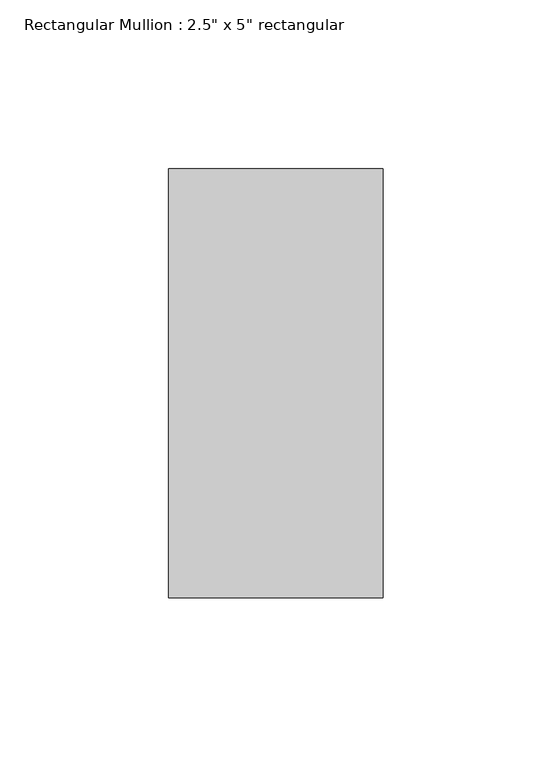
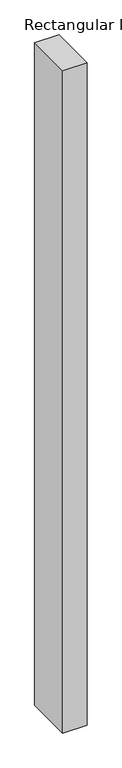
"""IFC4 building model written with IfcOpenShell, lengths in millimetres: member geometry."""

from ifc_helpers import new_model, si_unit, frame, origin, place, context, project, spatial, polyline, outline, extrude, source, transform, mapped, element, save


def member_163b98ee(model_context):
    return source(origin(), model_context, "Body", "SweptSolid", [
        extrude(outline(polyline([(31.75, 63.5), (31.75, -63.5), (-31.75, -63.5), (-31.75, 63.5), (31.75, 63.5)])), frame((0.0, 0.0, -1835.15), z_axis=(0.0, 0.0, 1.0), x_axis=(1.0, 0.0, 0.0)), (0.0, 0.0, 1.0), 1835.15),
    ])


if __name__ == "__main__":
    model = new_model("IFC4")
    model_context = context("Model", 3, world=origin())
    ifc_project = project(units=[si_unit("LENGTHUNIT", "METRE", prefix="MILLI")], contexts=[model_context])
    site = spatial("IfcSite", under=ifc_project)
    building = spatial("IfcBuilding", under=site)
    placement = place(None, origin())
    member_shape = member_163b98ee(model_context)
    element("IfcMember", 1, ObjectType="Rectangular Mullion : 2.5\" x 5\" rectangular", at=placement, inside=building, context=model_context, shape_type="MappedRepresentation", body=[
        mapped(member_shape, transform((0.0, 0.0, 0.0), x_axis=(1.0, 0.0, 0.0), y_axis=(0.0, 1.0, 0.0), z_axis=(0.0, 0.0, 1.0))),
    ])
    save(model, "model.ifc")

# Revit data of these elements
# Type "Rectangular Mullion : 2.5\" x 5\" rectangular"
#   built-in parameter 1007304 = 0.416667 (stored number, unit not read)
#   built-in parameter 1007301 = 0.104167 (stored number, unit not read)
#   built-in parameter 1007300 = 0.104167 (stored number, unit not read)
# Element 1 (IfcMember, "Rectangular Mullion : 2.5\" x 5\" rectangular")
#   Materials on its faces: "Aluminum"
# Materials
#   "Aluminum": class "Metal", colour RGB 247 247 247, transparency 0, Description = "Aluminum 6061", Cost = 0
